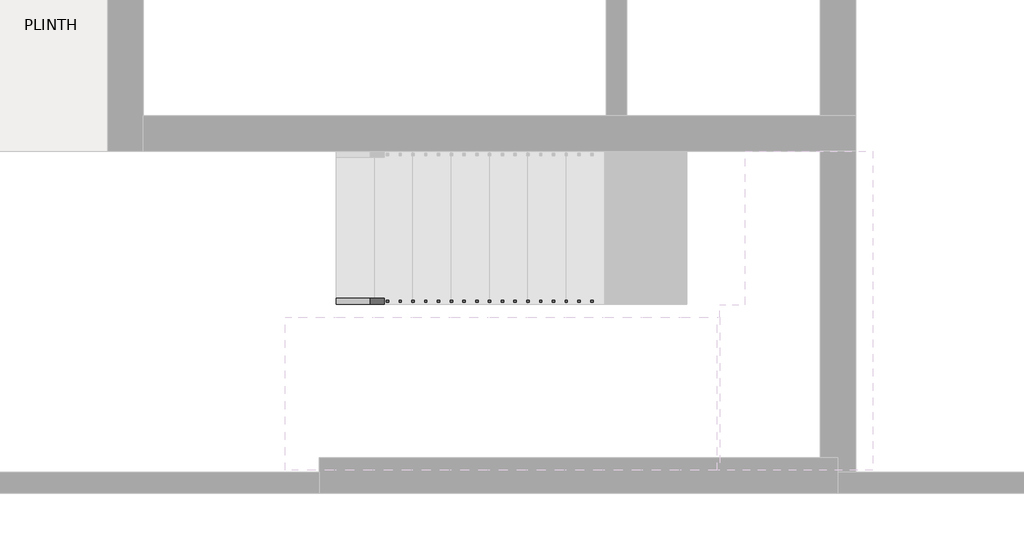
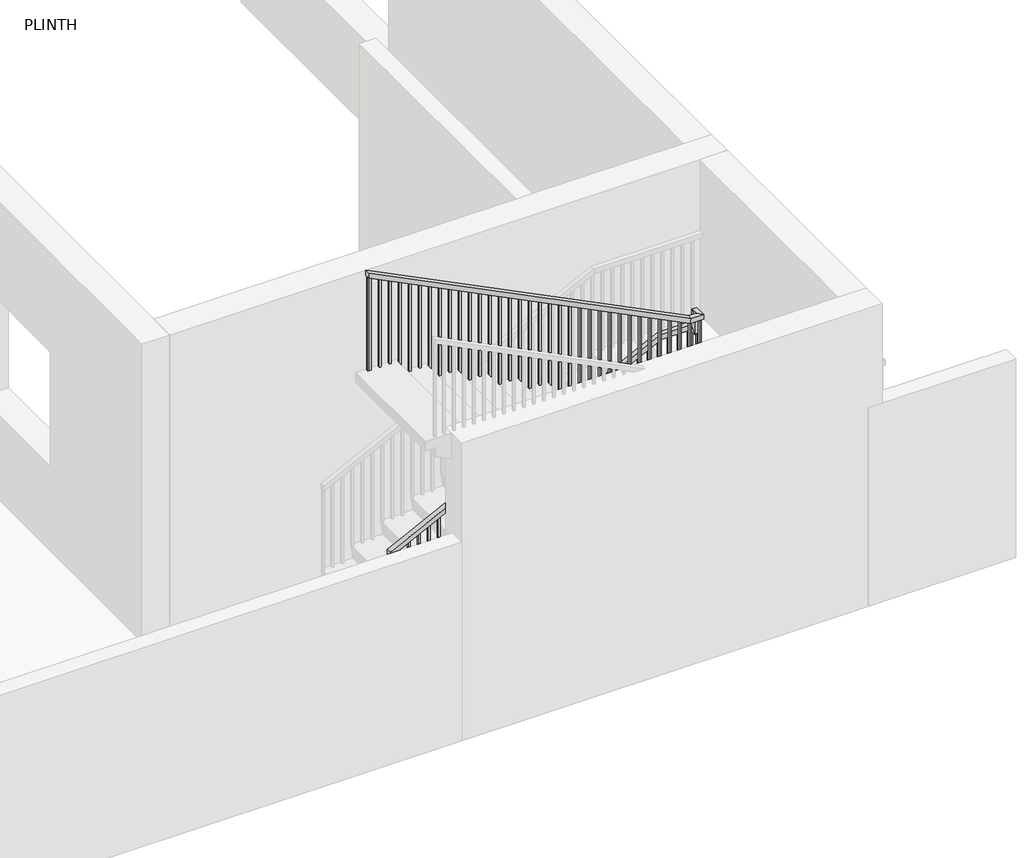
# One storey, part 2 of 3: 1 railing.
"""IFC4 building model written with IfcOpenShell, lengths in millimetres."""

from ifc_helpers import new_model, si_unit, frame, origin, place, context, project, spatial, polyline, outline, extrude, faceted_brep, element, save

model = new_model("IFC4")

# Units and contexts
model_context = context("Model", 3, world=origin())
ifc_project = project(units=[si_unit("LENGTHUNIT", "METRE", prefix="MILLI")], contexts=[model_context])

# Site, building, storey
site = spatial("IfcSite", under=ifc_project)
building = spatial("IfcBuilding", under=site)
storey = spatial("IfcBuildingStorey", under=building, Name="PLINTH", Elevation=0.0)

# Railing
placement = place(None, origin())
element("IfcRailing", 1, ObjectType="Handrail - Rectangular", at=placement, inside=storey, context=model_context, shape_type="SolidModel", body=[
    faceted_brep([(-13267.32252, -3954.8806156, 1066.8), (-13267.32252, -3954.8806156, 1010.0038734), (-13267.32252, -4005.6806156, 1010.0038734), (-13267.32252, -4005.6806156, 1066.8), (-10524.12252, -3954.8806156, 2438.4), (-10512.1302667, -3954.8806156, 2387.6), (-10512.1302667, -4005.6806156, 2387.6), (-10524.12252, -4005.6806156, 2438.4), (-10168.52252, -3954.8806156, 2438.4), (-10168.52252, -3954.8806156, 2387.6), (-10219.32252, -4005.6806156, 2387.6), (-10219.32252, -4005.6806156, 2438.4), (-10168.52252, -4031.0806156, 2438.4), (-10168.52252, -4081.8806156, 2387.6), (-10219.32252, -4081.8806156, 2387.6), (-10219.32252, -4031.0806156, 2438.4), (-10168.52252, -4031.0806156, 2628.9), (-10168.52252, -4081.8806156, 2578.1), (-10219.32252, -4081.8806156, 2578.1), (-10219.32252, -4031.0806156, 2628.9), (-10168.52252, -4158.0806156, 2628.9), (-10168.52252, -4158.0806156, 2578.1), (-10219.32252, -4107.2806156, 2578.1), (-10219.32252, -4107.2806156, 2628.9), (-10295.52252, -4158.0806156, 2628.9), (-10307.5147732, -4158.0806156, 2578.1), (-10307.5147732, -4107.2806156, 2578.1), (-10295.52252, -4107.2806156, 2628.9), (-13572.12252, -4158.0806156, 4267.2), (-13572.12252, -4107.2806156, 4267.2), (-13572.12252, -4107.2806156, 4210.4038734), (-13572.12252, -4158.0806156, 4210.4038734)], [[[0, 1, 2, 3]], [[1, 0, 4, 5]], [[2, 1, 5, 6]], [[3, 2, 6, 7]], [[0, 3, 7, 4]], [[5, 4, 8, 9]], [[6, 5, 9, 10]], [[7, 6, 10, 11]], [[4, 7, 11, 8]], [[9, 8, 12, 13]], [[10, 9, 13, 14]], [[11, 10, 14, 15]], [[8, 11, 15, 12]], [[13, 12, 16, 17]], [[14, 13, 17, 18]], [[15, 14, 18, 19]], [[12, 15, 19, 16]], [[17, 16, 20, 21]], [[18, 17, 21, 22]], [[19, 18, 22, 23]], [[16, 19, 23, 20]], [[21, 20, 24, 25]], [[22, 21, 25, 26]], [[23, 22, 26, 27]], [[20, 23, 27, 24]], [[28, 29, 30, 31]], [[25, 24, 28, 31]], [[26, 25, 31, 30]], [[27, 26, 30, 29]], [[24, 27, 29, 28]]]),
    extrude(outline(polyline([(4192.9413734, -13537.19752), (4202.4663734, -13556.24752), (3200.4, -13556.24752), (3200.4, -13537.19752), (4192.9413734, -13537.19752)])), frame((0.0, -4142.2056156, 0.0), z_axis=(0.0, 1.0, 0.0), x_axis=(0.0, 0.0, 1.0)), (0.0, 0.0, 1.0), 19.05),
    extrude(outline(polyline([(4142.1413734, -13435.59752), (4151.6663734, -13454.64752), (3200.4, -13454.64752), (3200.4, -13435.59752), (4142.1413734, -13435.59752)])), frame((0.0, -4142.2056156, 0.0), z_axis=(0.0, 1.0, 0.0), x_axis=(0.0, 0.0, 1.0)), (0.0, 0.0, 1.0), 19.05),
    extrude(outline(polyline([(4091.3413734, -13333.99752), (4100.8663734, -13353.04752), (3200.4, -13353.04752), (3200.4, -13333.99752), (4091.3413734, -13333.99752)])), frame((0.0, -4142.2056156, 0.0), z_axis=(0.0, 1.0, 0.0), x_axis=(0.0, 0.0, 1.0)), (0.0, 0.0, 1.0), 19.05),
    extrude(outline(polyline([(4040.5413734, -13232.39752), (4050.0663734, -13251.44752), (3048.0, -13251.44752), (3048.0, -13232.39752), (4040.5413734, -13232.39752)])), frame((0.0, -4142.2056156, 0.0), z_axis=(0.0, 1.0, 0.0), x_axis=(0.0, 0.0, 1.0)), (0.0, 0.0, 1.0), 19.05),
    extrude(outline(polyline([(3989.7413734, -13130.79752), (3999.2663734, -13149.84752), (3048.0, -13149.84752), (3048.0, -13130.79752), (3989.7413734, -13130.79752)])), frame((0.0, -4142.2056156, 0.0), z_axis=(0.0, 1.0, 0.0), x_axis=(0.0, 0.0, 1.0)), (0.0, 0.0, 1.0), 19.05),
    extrude(outline(polyline([(3938.9413734, -13029.19752), (3948.4663734, -13048.24752), (3048.0, -13048.24752), (3048.0, -13029.19752), (3938.9413734, -13029.19752)])), frame((0.0, -4142.2056156, 0.0), z_axis=(0.0, 1.0, 0.0), x_axis=(0.0, 0.0, 1.0)), (0.0, 0.0, 1.0), 19.05),
    extrude(outline(polyline([(3888.1413734, -12927.59752), (3897.6663734, -12946.64752), (2895.6, -12946.64752), (2895.6, -12927.59752), (3888.1413734, -12927.59752)])), frame((0.0, -4142.2056156, 0.0), z_axis=(0.0, 1.0, 0.0), x_axis=(0.0, 0.0, 1.0)), (0.0, 0.0, 1.0), 19.05),
    extrude(outline(polyline([(3837.3413734, -12825.99752), (3846.8663734, -12845.04752), (2895.6, -12845.04752), (2895.6, -12825.99752), (3837.3413734, -12825.99752)])), frame((0.0, -4142.2056156, 0.0), z_axis=(0.0, 1.0, 0.0), x_axis=(0.0, 0.0, 1.0)), (0.0, 0.0, 1.0), 19.05),
    extrude(outline(polyline([(3786.5413734, -12724.39752), (3796.0663734, -12743.44752), (2895.6, -12743.44752), (2895.6, -12724.39752), (3786.5413734, -12724.39752)])), frame((0.0, -4142.2056156, 0.0), z_axis=(0.0, 1.0, 0.0), x_axis=(0.0, 0.0, 1.0)), (0.0, 0.0, 1.0), 19.05),
    extrude(outline(polyline([(3735.7413734, -12622.79752), (3745.2663734, -12641.84752), (2743.2, -12641.84752), (2743.2, -12622.79752), (3735.7413734, -12622.79752)])), frame((0.0, -4142.2056156, 0.0), z_axis=(0.0, 1.0, 0.0), x_axis=(0.0, 0.0, 1.0)), (0.0, 0.0, 1.0), 19.05),
    extrude(outline(polyline([(3684.9413734, -12521.19752), (3694.4663734, -12540.24752), (2743.2, -12540.24752), (2743.2, -12521.19752), (3684.9413734, -12521.19752)])), frame((0.0, -4142.2056156, 0.0), z_axis=(0.0, 1.0, 0.0), x_axis=(0.0, 0.0, 1.0)), (0.0, 0.0, 1.0), 19.05),
    extrude(outline(polyline([(3634.1413734, -12419.59752), (3643.6663734, -12438.64752), (2743.2, -12438.64752), (2743.2, -12419.59752), (3634.1413734, -12419.59752)])), frame((0.0, -4142.2056156, 0.0), z_axis=(0.0, 1.0, 0.0), x_axis=(0.0, 0.0, 1.0)), (0.0, 0.0, 1.0), 19.05),
    extrude(outline(polyline([(3583.3413734, -12317.99752), (3592.8663734, -12337.04752), (2590.8, -12337.04752), (2590.8, -12317.99752), (3583.3413734, -12317.99752)])), frame((0.0, -4142.2056156, 0.0), z_axis=(0.0, 1.0, 0.0), x_axis=(0.0, 0.0, 1.0)), (0.0, 0.0, 1.0), 19.05),
    extrude(outline(polyline([(3532.5413734, -12216.39752), (3542.0663734, -12235.44752), (2590.8, -12235.44752), (2590.8, -12216.39752), (3532.5413734, -12216.39752)])), frame((0.0, -4142.2056156, 0.0), z_axis=(0.0, 1.0, 0.0), x_axis=(0.0, 0.0, 1.0)), (0.0, 0.0, 1.0), 19.05),
    extrude(outline(polyline([(3481.7413734, -12114.79752), (3491.2663734, -12133.84752), (2590.8, -12133.84752), (2590.8, -12114.79752), (3481.7413734, -12114.79752)])), frame((0.0, -4142.2056156, 0.0), z_axis=(0.0, 1.0, 0.0), x_axis=(0.0, 0.0, 1.0)), (0.0, 0.0, 1.0), 19.05),
    extrude(outline(polyline([(3430.9413734, -12013.19752), (3440.4663734, -12032.24752), (2438.4, -12032.24752), (2438.4, -12013.19752), (3430.9413734, -12013.19752)])), frame((0.0, -4142.2056156, 0.0), z_axis=(0.0, 1.0, 0.0), x_axis=(0.0, 0.0, 1.0)), (0.0, 0.0, 1.0), 19.05),
    extrude(outline(polyline([(3380.1413734, -11911.59752), (3389.6663734, -11930.64752), (2438.4, -11930.64752), (2438.4, -11911.59752), (3380.1413734, -11911.59752)])), frame((0.0, -4142.2056156, 0.0), z_axis=(0.0, 1.0, 0.0), x_axis=(0.0, 0.0, 1.0)), (0.0, 0.0, 1.0), 19.05),
    extrude(outline(polyline([(3329.3413734, -11809.99752), (3338.8663734, -11829.04752), (2438.4, -11829.04752), (2438.4, -11809.99752), (3329.3413734, -11809.99752)])), frame((0.0, -4142.2056156, 0.0), z_axis=(0.0, 1.0, 0.0), x_axis=(0.0, 0.0, 1.0)), (0.0, 0.0, 1.0), 19.05),
    extrude(outline(polyline([(3278.5413734, -11708.39752), (3288.0663734, -11727.44752), (2286.0, -11727.44752), (2286.0, -11708.39752), (3278.5413734, -11708.39752)])), frame((0.0, -4142.2056156, 0.0), z_axis=(0.0, 1.0, 0.0), x_axis=(0.0, 0.0, 1.0)), (0.0, 0.0, 1.0), 19.05),
    extrude(outline(polyline([(3227.7413734, -11606.79752), (3237.2663734, -11625.84752), (2286.0, -11625.84752), (2286.0, -11606.79752), (3227.7413734, -11606.79752)])), frame((0.0, -4142.2056156, 0.0), z_axis=(0.0, 1.0, 0.0), x_axis=(0.0, 0.0, 1.0)), (0.0, 0.0, 1.0), 19.05),
    extrude(outline(polyline([(3176.9413734, -11505.19752), (3186.4663734, -11524.24752), (2286.0, -11524.24752), (2286.0, -11505.19752), (3176.9413734, -11505.19752)])), frame((0.0, -4142.2056156, 0.0), z_axis=(0.0, 1.0, 0.0), x_axis=(0.0, 0.0, 1.0)), (0.0, 0.0, 1.0), 19.05),
    extrude(outline(polyline([(3126.1413734, -11403.59752), (3135.6663734, -11422.64752), (2133.6, -11422.64752), (2133.6, -11403.59752), (3126.1413734, -11403.59752)])), frame((0.0, -4142.2056156, 0.0), z_axis=(0.0, 1.0, 0.0), x_axis=(0.0, 0.0, 1.0)), (0.0, 0.0, 1.0), 19.05),
    extrude(outline(polyline([(3075.3413734, -11301.99752), (3084.8663734, -11321.04752), (2133.6, -11321.04752), (2133.6, -11301.99752), (3075.3413734, -11301.99752)])), frame((0.0, -4142.2056156, 0.0), z_axis=(0.0, 1.0, 0.0), x_axis=(0.0, 0.0, 1.0)), (0.0, 0.0, 1.0), 19.05),
    extrude(outline(polyline([(3024.5413734, -11200.39752), (3034.0663734, -11219.44752), (2133.6, -11219.44752), (2133.6, -11200.39752), (3024.5413734, -11200.39752)])), frame((0.0, -4142.2056156, 0.0), z_axis=(0.0, 1.0, 0.0), x_axis=(0.0, 0.0, 1.0)), (0.0, 0.0, 1.0), 19.05),
    extrude(outline(polyline([(2973.7413734, -11098.79752), (2983.2663734, -11117.84752), (1981.2, -11117.84752), (1981.2, -11098.79752), (2973.7413734, -11098.79752)])), frame((0.0, -4142.2056156, 0.0), z_axis=(0.0, 1.0, 0.0), x_axis=(0.0, 0.0, 1.0)), (0.0, 0.0, 1.0), 19.05),
    extrude(outline(polyline([(2922.9413734, -10997.19752), (2932.4663734, -11016.24752), (1981.2, -11016.24752), (1981.2, -10997.19752), (2922.9413734, -10997.19752)])), frame((0.0, -4142.2056156, 0.0), z_axis=(0.0, 1.0, 0.0), x_axis=(0.0, 0.0, 1.0)), (0.0, 0.0, 1.0), 19.05),
    extrude(outline(polyline([(2872.1413734, -10895.59752), (2881.6663734, -10914.64752), (1981.2, -10914.64752), (1981.2, -10895.59752), (2872.1413734, -10895.59752)])), frame((0.0, -4142.2056156, 0.0), z_axis=(0.0, 1.0, 0.0), x_axis=(0.0, 0.0, 1.0)), (0.0, 0.0, 1.0), 19.05),
    extrude(outline(polyline([(2821.3413734, -10793.99752), (2830.8663734, -10813.04752), (1828.8, -10813.04752), (1828.8, -10793.99752), (2821.3413734, -10793.99752)])), frame((0.0, -4142.2056156, 0.0), z_axis=(0.0, 1.0, 0.0), x_axis=(0.0, 0.0, 1.0)), (0.0, 0.0, 1.0), 19.05),
    extrude(outline(polyline([(2770.5413734, -10692.39752), (2780.0663734, -10711.44752), (1828.8, -10711.44752), (1828.8, -10692.39752), (2770.5413734, -10692.39752)])), frame((0.0, -4142.2056156, 0.0), z_axis=(0.0, 1.0, 0.0), x_axis=(0.0, 0.0, 1.0)), (0.0, 0.0, 1.0), 19.05),
    extrude(outline(polyline([(2719.7413734, -10590.79752), (2729.2663734, -10609.84752), (1828.8, -10609.84752), (1828.8, -10590.79752), (2719.7413734, -10590.79752)])), frame((0.0, -4142.2056156, 0.0), z_axis=(0.0, 1.0, 0.0), x_axis=(0.0, 0.0, 1.0)), (0.0, 0.0, 1.0), 19.05),
    extrude(outline(polyline([(2668.9413734, -10489.19752), (2678.4663734, -10508.24752), (1676.4, -10508.24752), (1676.4, -10489.19752), (2668.9413734, -10489.19752)])), frame((0.0, -4142.2056156, 0.0), z_axis=(0.0, 1.0, 0.0), x_axis=(0.0, 0.0, 1.0)), (0.0, 0.0, 1.0), 19.05),
    extrude(outline(polyline([(2618.1413734, -10387.59752), (2627.6663734, -10406.64752), (1676.4, -10406.64752), (1676.4, -10387.59752), (2618.1413734, -10387.59752)])), frame((0.0, -4142.2056156, 0.0), z_axis=(0.0, 1.0, 0.0), x_axis=(0.0, 0.0, 1.0)), (0.0, 0.0, 1.0), 19.05),
    extrude(outline(polyline([(-10285.99752, -4123.1556156), (-10285.99752, -4142.2056156), (-10305.04752, -4142.2056156), (-10305.04752, -4123.1556156), (-10285.99752, -4123.1556156)])), frame((0.0, 0.0, 1676.4), z_axis=(0.0, 0.0, 1.0), x_axis=(1.0, 0.0, 0.0)), (0.0, 0.0, 1.0), 901.7),
    extrude(outline(polyline([(-10203.44752, -4072.3556156), (-10184.39752, -4072.3556156), (-10184.39752, -4091.4056156), (-10203.44752, -4091.4056156), (-10203.44752, -4072.3556156)])), frame((0.0, 0.0, 1524.0), z_axis=(0.0, 0.0, 1.0), x_axis=(1.0, 0.0, 0.0)), (0.0, 0.0, 1.0), 863.6),
    extrude(outline(polyline([(-10228.84752, -3989.8056156), (-10228.84752, -3970.7556156), (-10209.79752, -3970.7556156), (-10209.79752, -3989.8056156), (-10228.84752, -3989.8056156)])), frame((0.0, 0.0, 1524.0), z_axis=(0.0, 0.0, 1.0), x_axis=(1.0, 0.0, 0.0)), (0.0, 0.0, 1.0), 863.6),
    extrude(outline(polyline([(-10330.44752, -3989.8056156), (-10330.44752, -3970.7556156), (-10311.39752, -3970.7556156), (-10311.39752, -3989.8056156), (-10330.44752, -3989.8056156)])), frame((0.0, 0.0, 1524.0), z_axis=(0.0, 0.0, 1.0), x_axis=(1.0, 0.0, 0.0)), (0.0, 0.0, 1.0), 863.6),
    extrude(outline(polyline([(-10432.04752, -3989.8056156), (-10432.04752, -3970.7556156), (-10412.99752, -3970.7556156), (-10412.99752, -3989.8056156), (-10432.04752, -3989.8056156)])), frame((0.0, 0.0, 1524.0), z_axis=(0.0, 0.0, 1.0), x_axis=(1.0, 0.0, 0.0)), (0.0, 0.0, 1.0), 863.6),
    extrude(outline(polyline([(2335.5663734, -10616.19752), (2326.0413734, -10635.24752), (1371.6, -10635.24752), (1371.6, -10616.19752), (2335.5663734, -10616.19752)])), frame((0.0, -3989.8056156, 0.0), z_axis=(0.0, 1.0, 0.0), x_axis=(0.0, 0.0, 1.0)), (0.0, 0.0, 1.0), 19.05),
    extrude(outline(polyline([(2284.7663734, -10717.79752), (2275.2413734, -10736.84752), (1371.6, -10736.84752), (1371.6, -10717.79752), (2284.7663734, -10717.79752)])), frame((0.0, -3989.8056156, 0.0), z_axis=(0.0, 1.0, 0.0), x_axis=(0.0, 0.0, 1.0)), (0.0, 0.0, 1.0), 19.05),
    extrude(outline(polyline([(2233.9663734, -10819.39752), (2224.4413734, -10838.44752), (1371.6, -10838.44752), (1371.6, -10819.39752), (2233.9663734, -10819.39752)])), frame((0.0, -3989.8056156, 0.0), z_axis=(0.0, 1.0, 0.0), x_axis=(0.0, 0.0, 1.0)), (0.0, 0.0, 1.0), 19.05),
    extrude(outline(polyline([(2183.1663734, -10920.99752), (2173.6413734, -10940.04752), (1219.2, -10940.04752), (1219.2, -10920.99752), (2183.1663734, -10920.99752)])), frame((0.0, -3989.8056156, 0.0), z_axis=(0.0, 1.0, 0.0), x_axis=(0.0, 0.0, 1.0)), (0.0, 0.0, 1.0), 19.05),
    extrude(outline(polyline([(2132.3663734, -11022.59752), (2122.8413734, -11041.64752), (1219.2, -11041.64752), (1219.2, -11022.59752), (2132.3663734, -11022.59752)])), frame((0.0, -3989.8056156, 0.0), z_axis=(0.0, 1.0, 0.0), x_axis=(0.0, 0.0, 1.0)), (0.0, 0.0, 1.0), 19.05),
    extrude(outline(polyline([(2081.5663734, -11124.19752), (2072.0413734, -11143.24752), (1219.2, -11143.24752), (1219.2, -11124.19752), (2081.5663734, -11124.19752)])), frame((0.0, -3989.8056156, 0.0), z_axis=(0.0, 1.0, 0.0), x_axis=(0.0, 0.0, 1.0)), (0.0, 0.0, 1.0), 19.05),
    extrude(outline(polyline([(2030.7663734, -11225.79752), (2021.2413734, -11244.84752), (1066.8, -11244.84752), (1066.8, -11225.79752), (2030.7663734, -11225.79752)])), frame((0.0, -3989.8056156, 0.0), z_axis=(0.0, 1.0, 0.0), x_axis=(0.0, 0.0, 1.0)), (0.0, 0.0, 1.0), 19.05),
    extrude(outline(polyline([(1979.9663734, -11327.39752), (1970.4413734, -11346.44752), (1066.8, -11346.44752), (1066.8, -11327.39752), (1979.9663734, -11327.39752)])), frame((0.0, -3989.8056156, 0.0), z_axis=(0.0, 1.0, 0.0), x_axis=(0.0, 0.0, 1.0)), (0.0, 0.0, 1.0), 19.05),
    extrude(outline(polyline([(1929.1663734, -11428.99752), (1919.6413734, -11448.04752), (1066.8, -11448.04752), (1066.8, -11428.99752), (1929.1663734, -11428.99752)])), frame((0.0, -3989.8056156, 0.0), z_axis=(0.0, 1.0, 0.0), x_axis=(0.0, 0.0, 1.0)), (0.0, 0.0, 1.0), 19.05),
    extrude(outline(polyline([(1878.3663734, -11530.59752), (1868.8413734, -11549.64752), (914.4, -11549.64752), (914.4, -11530.59752), (1878.3663734, -11530.59752)])), frame((0.0, -3989.8056156, 0.0), z_axis=(0.0, 1.0, 0.0), x_axis=(0.0, 0.0, 1.0)), (0.0, 0.0, 1.0), 19.05),
    extrude(outline(polyline([(1827.5663734, -11632.19752), (1818.0413734, -11651.24752), (914.4, -11651.24752), (914.4, -11632.19752), (1827.5663734, -11632.19752)])), frame((0.0, -3989.8056156, 0.0), z_axis=(0.0, 1.0, 0.0), x_axis=(0.0, 0.0, 1.0)), (0.0, 0.0, 1.0), 19.05),
    extrude(outline(polyline([(1776.7663734, -11733.79752), (1767.2413734, -11752.84752), (914.4, -11752.84752), (914.4, -11733.79752), (1776.7663734, -11733.79752)])), frame((0.0, -3989.8056156, 0.0), z_axis=(0.0, 1.0, 0.0), x_axis=(0.0, 0.0, 1.0)), (0.0, 0.0, 1.0), 19.05),
    extrude(outline(polyline([(1725.9663734, -11835.39752), (1716.4413734, -11854.44752), (762.0, -11854.44752), (762.0, -11835.39752), (1725.9663734, -11835.39752)])), frame((0.0, -3989.8056156, 0.0), z_axis=(0.0, 1.0, 0.0), x_axis=(0.0, 0.0, 1.0)), (0.0, 0.0, 1.0), 19.05),
    extrude(outline(polyline([(1675.1663734, -11936.99752), (1665.6413734, -11956.04752), (762.0, -11956.04752), (762.0, -11936.99752), (1675.1663734, -11936.99752)])), frame((0.0, -3989.8056156, 0.0), z_axis=(0.0, 1.0, 0.0), x_axis=(0.0, 0.0, 1.0)), (0.0, 0.0, 1.0), 19.05),
    extrude(outline(polyline([(1624.3663734, -12038.59752), (1614.8413734, -12057.64752), (762.0, -12057.64752), (762.0, -12038.59752), (1624.3663734, -12038.59752)])), frame((0.0, -3989.8056156, 0.0), z_axis=(0.0, 1.0, 0.0), x_axis=(0.0, 0.0, 1.0)), (0.0, 0.0, 1.0), 19.05),
    extrude(outline(polyline([(1573.5663734, -12140.19752), (1564.0413734, -12159.24752), (609.6, -12159.24752), (609.6, -12140.19752), (1573.5663734, -12140.19752)])), frame((0.0, -3989.8056156, 0.0), z_axis=(0.0, 1.0, 0.0), x_axis=(0.0, 0.0, 1.0)), (0.0, 0.0, 1.0), 19.05),
    extrude(outline(polyline([(1522.7663734, -12241.79752), (1513.2413734, -12260.84752), (609.6, -12260.84752), (609.6, -12241.79752), (1522.7663734, -12241.79752)])), frame((0.0, -3989.8056156, 0.0), z_axis=(0.0, 1.0, 0.0), x_axis=(0.0, 0.0, 1.0)), (0.0, 0.0, 1.0), 19.05),
    extrude(outline(polyline([(1471.9663734, -12343.39752), (1462.4413734, -12362.44752), (609.6, -12362.44752), (609.6, -12343.39752), (1471.9663734, -12343.39752)])), frame((0.0, -3989.8056156, 0.0), z_axis=(0.0, 1.0, 0.0), x_axis=(0.0, 0.0, 1.0)), (0.0, 0.0, 1.0), 19.05),
    extrude(outline(polyline([(1421.1663734, -12444.99752), (1411.6413734, -12464.04752), (457.2, -12464.04752), (457.2, -12444.99752), (1421.1663734, -12444.99752)])), frame((0.0, -3989.8056156, 0.0), z_axis=(0.0, 1.0, 0.0), x_axis=(0.0, 0.0, 1.0)), (0.0, 0.0, 1.0), 19.05),
    extrude(outline(polyline([(1370.3663734, -12546.59752), (1360.8413734, -12565.64752), (457.2, -12565.64752), (457.2, -12546.59752), (1370.3663734, -12546.59752)])), frame((0.0, -3989.8056156, 0.0), z_axis=(0.0, 1.0, 0.0), x_axis=(0.0, 0.0, 1.0)), (0.0, 0.0, 1.0), 19.05),
    extrude(outline(polyline([(1319.5663734, -12648.19752), (1310.0413734, -12667.24752), (457.2, -12667.24752), (457.2, -12648.19752), (1319.5663734, -12648.19752)])), frame((0.0, -3989.8056156, 0.0), z_axis=(0.0, 1.0, 0.0), x_axis=(0.0, 0.0, 1.0)), (0.0, 0.0, 1.0), 19.05),
    extrude(outline(polyline([(1268.7663734, -12749.79752), (1259.2413734, -12768.84752), (304.8, -12768.84752), (304.8, -12749.79752), (1268.7663734, -12749.79752)])), frame((0.0, -3989.8056156, 0.0), z_axis=(0.0, 1.0, 0.0), x_axis=(0.0, 0.0, 1.0)), (0.0, 0.0, 1.0), 19.05),
    extrude(outline(polyline([(1217.9663734, -12851.39752), (1208.4413734, -12870.44752), (304.8, -12870.44752), (304.8, -12851.39752), (1217.9663734, -12851.39752)])), frame((0.0, -3989.8056156, 0.0), z_axis=(0.0, 1.0, 0.0), x_axis=(0.0, 0.0, 1.0)), (0.0, 0.0, 1.0), 19.05),
    extrude(outline(polyline([(1167.1663734, -12952.99752), (1157.6413734, -12972.04752), (304.8, -12972.04752), (304.8, -12952.99752), (1167.1663734, -12952.99752)])), frame((0.0, -3989.8056156, 0.0), z_axis=(0.0, 1.0, 0.0), x_axis=(0.0, 0.0, 1.0)), (0.0, 0.0, 1.0), 19.05),
    extrude(outline(polyline([(1116.3663734, -13054.59752), (1106.8413734, -13073.64752), (152.4, -13073.64752), (152.4, -13054.59752), (1116.3663734, -13054.59752)])), frame((0.0, -3989.8056156, 0.0), z_axis=(0.0, 1.0, 0.0), x_axis=(0.0, 0.0, 1.0)), (0.0, 0.0, 1.0), 19.05),
    extrude(outline(polyline([(1065.5663734, -13156.19752), (1056.0413734, -13175.24752), (152.4, -13175.24752), (152.4, -13156.19752), (1065.5663734, -13156.19752)])), frame((0.0, -3989.8056156, 0.0), z_axis=(0.0, 1.0, 0.0), x_axis=(0.0, 0.0, 1.0)), (0.0, 0.0, 1.0), 19.05),
    extrude(outline(polyline([(-10184.39752, -4123.1556156), (-10184.39752, -4142.2056156), (-10203.44752, -4142.2056156), (-10203.44752, -4123.1556156), (-10184.39752, -4123.1556156)])), frame((0.0, 0.0, 1524.0), z_axis=(0.0, 0.0, 1.0), x_axis=(1.0, 0.0, 0.0)), (0.0, 0.0, 1.0), 1054.1),
    extrude(outline(polyline([(-10203.44752, -3989.8056156), (-10203.44752, -3970.7556156), (-10184.39752, -3970.7556156), (-10184.39752, -3989.8056156), (-10203.44752, -3989.8056156)])), frame((0.0, 0.0, 1524.0), z_axis=(0.0, 0.0, 1.0), x_axis=(1.0, 0.0, 0.0)), (0.0, 0.0, 1.0), 863.6),
    extrude(outline(polyline([(2386.3663734, -10514.59752), (2376.8413734, -10533.64752), (1524.0, -10533.64752), (1524.0, -10514.59752), (2386.3663734, -10514.59752)])), frame((0.0, -3989.8056156, 0.0), z_axis=(0.0, 1.0, 0.0), x_axis=(0.0, 0.0, 1.0)), (0.0, 0.0, 1.0), 19.05),
    extrude(outline(polyline([(4200.8788734, -13553.07252), (4210.4038734, -13572.12252), (3200.4, -13572.12252), (3200.4, -13553.07252), (4200.8788734, -13553.07252)])), frame((0.0, -4142.2056156, 0.0), z_axis=(0.0, 1.0, 0.0), x_axis=(0.0, 0.0, 1.0)), (0.0, 0.0, 1.0), 19.05),
    extrude(outline(polyline([(1019.5288734, -13248.27252), (1010.0038734, -13267.32252), (152.4, -13267.32252), (152.4, -13248.27252), (1019.5288734, -13248.27252)])), frame((0.0, -3989.8056156, 0.0), z_axis=(0.0, 1.0, 0.0), x_axis=(0.0, 0.0, 1.0)), (0.0, 0.0, 1.0), 19.05),
])

save(model, "model.ifc")

# Revit data of these elements
# Type "Handrail - Rectangular"
#   Assembly Code = "C2010400"
#   built-in parameter 1008612 = 0.0416667 (stored number, unit not read)
#   built-in parameter 1008611 = 0.0416667 (stored number, unit not read)
#   built-in parameter 1008609 = 0.333333 (stored number, unit not read)
#   built-in parameter 1008604 = 0.166667 (stored number, unit not read)
#   built-in parameter 1008603 = 0.166667 (stored number, unit not read)
#   Railing Height = 3' - 0"
#   built-in parameter 1008630 = 2
#   built-in parameter 1008610 = 2
#   built-in parameter 1008618 = Baluster - Square : 3/4"
# Element 1 (IfcRailing, "Handrail - Rectangular")
#   Phase Created = New Construction
